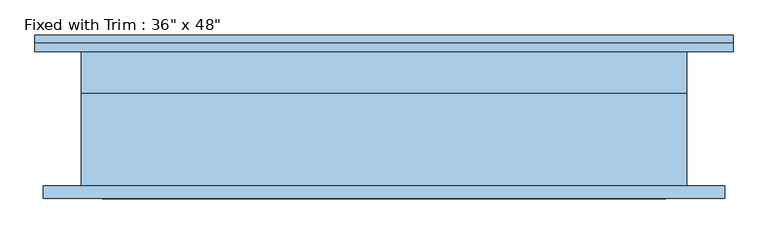
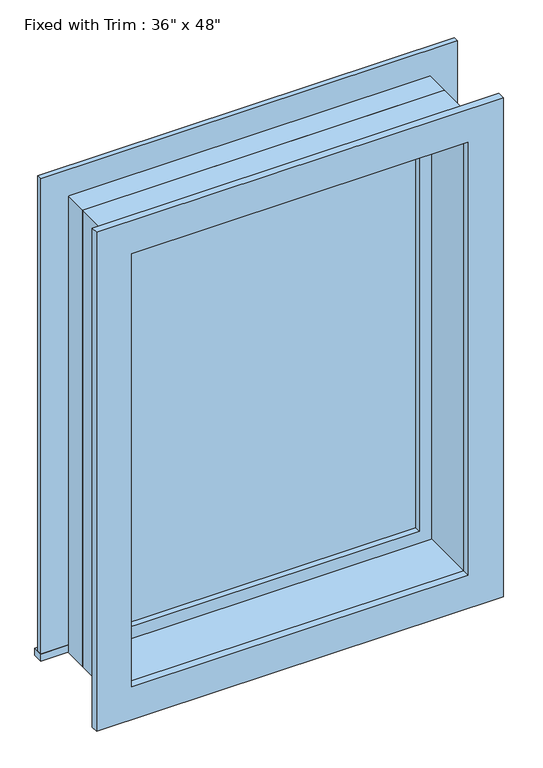
"""IFC4 building model written with IfcOpenShell, lengths in millimetres: window geometry."""

from ifc_helpers import new_model, si_unit, frame, origin, place, context, project, spatial, polyline, outline, extrude, source, transform, mapped, element, save


def window_bec2521a(model_context):
    return source(origin(), model_context, "Body", "SweptSolid", [
        extrude(outline(polyline([(-565.15, 127.0), (488.95, 127.0), (488.95, 101.6), (-565.15, 101.6), (-565.15, 127.0)])), frame((0.0, 0.0, 914.4), z_axis=(0.0, 0.0, 1.0), x_axis=(1.0, 0.0, 0.0)), (0.0, 0.0, 1.0), 19.05),
        extrude(outline(polyline([(2114.55, -476.25), (2114.55, 400.05), (933.45, 400.05), (933.45, 488.95), (2203.45, 488.95), (2203.45, -565.15), (933.45, -565.15), (933.45, -476.25), (2114.55, -476.25)])), frame((0.0, 101.6, 0.0), z_axis=(0.0, 1.0, 0.0), x_axis=(0.0, 0.0, 1.0)), (0.0, 0.0, 1.0), 12.7),
        extrude(outline(polyline([(2190.75, 476.25), (2190.75, -552.45), (857.25, -552.45), (857.25, 476.25), (2190.75, 476.25)]), holes=[polyline([(2101.85, 387.35), (946.15, 387.35), (946.15, -463.55), (2101.85, -463.55), (2101.85, 387.35)])]), frame((0.0, -120.65, 0.0), z_axis=(0.0, 1.0, 0.0), x_axis=(0.0, 0.0, 1.0)), (0.0, 0.0, 1.0), 19.05),
        extrude(outline(polyline([(355.6, 53.975), (-431.8, 53.975), (-431.8, 66.675), (355.6, 66.675), (355.6, 53.975)])), frame((0.0, 0.0, 977.9), z_axis=(0.0, 0.0, 1.0), x_axis=(1.0, 0.0, 0.0)), (0.0, 0.0, 1.0), 1092.2),
        extrude(outline(polyline([(2114.55, -476.25), (933.45, -476.25), (933.45, 400.05), (2114.55, 400.05), (2114.55, -476.25)]), holes=[polyline([(2070.1, -431.8), (2070.1, 355.6), (977.9, 355.6), (977.9, -431.8), (2070.1, -431.8)])]), frame((0.0, 38.1, 0.0), z_axis=(0.0, 1.0, 0.0), x_axis=(0.0, 0.0, 1.0)), (0.0, 0.0, 1.0), 44.45),
        extrude(outline(polyline([(2133.6, -495.3), (914.4, -495.3), (914.4, 419.1), (2133.6, 419.1), (2133.6, -495.3)]), holes=[polyline([(2101.85, -463.55), (2101.85, 387.35), (946.15, 387.35), (946.15, -463.55), (2101.85, -463.55)])]), frame((0.0, -101.6, 0.0), z_axis=(0.0, 1.0, 0.0), x_axis=(0.0, 0.0, 1.0)), (0.0, 0.0, 1.0), 139.7),
        extrude(outline(polyline([(2133.6, 419.1), (2133.6, -495.3), (914.4, -495.3), (914.4, 419.1), (2133.6, 419.1)]), holes=[polyline([(2114.55, 400.05), (933.45, 400.05), (933.45, -476.25), (2114.55, -476.25), (2114.55, 400.05)])]), frame((0.0, 38.1, 0.0), z_axis=(0.0, 1.0, 0.0), x_axis=(0.0, 0.0, 1.0)), (0.0, 0.0, 1.0), 63.5),
    ])


if __name__ == "__main__":
    model = new_model("IFC4")
    model_context = context("Model", 3, world=origin())
    ifc_project = project(units=[si_unit("LENGTHUNIT", "METRE", prefix="MILLI")], contexts=[model_context])
    site = spatial("IfcSite", under=ifc_project)
    building = spatial("IfcBuilding", under=site)
    placement = place(None, origin())
    window_shape = window_bec2521a(model_context)
    element("IfcWindow", 1, ObjectType="Fixed with Trim : 36\" x 48\"", at=placement, inside=building, context=model_context, shape_type="MappedRepresentation", body=[
        mapped(window_shape, transform((0.0, 0.0, 0.0), x_axis=(1.0, 0.0, 0.0), y_axis=(0.0, 1.0, 0.0), z_axis=(0.0, 0.0, 1.0))),
    ])
    save(model, "model.ifc")

# Revit data of these elements
# Type "Fixed with Trim : 36\" x 48\""
#   Type Mark = "10"
#   Construction Type Id = "GSP4R"
#   Assembly Code = "B2020100"
#   Analytic Construction = "1/8 in Pilkington single glazing"
#   Visual Light Transmittance = 0.9
#   Solar Heat Gain Coefficient = 0.78
#   Heat Transfer Coefficient (U) = 0.6496 BTU/(h·ft²·°F)
#   Height = 4' - 0"
#   Default Sill Height = 3' - 0"
#   Trim Projection - Ext. = 0' - 0 1/2"
#   Trim Projection - Int. = 0' - 0 3/4"
#   Trim Width - Exterior = 0' - 3 1/2"
#   Trim Width - Interior = 0' - 3 1/2"
#   Width = 3' - 0"
#   Window Inset = 0' - 0 3/4"
#   Define Thermal Properties by = 1
#   Glass Pane Material = Glass
#   Sash Material = Sash
#   Trim Exterior Material = Trim
#   Trim Interior Material = Trim
#   Wall Closure = (empty or 0)
# Element 1 (IfcWindow, "Fixed with Trim : 36\" x 48\"")
#   Materials on its faces: "Sash", "Trim", "Glass"
# Materials
#   "Glass": class "Glass", colour RGB 0 128 192, transparency 0.75, Description = "Soda Lime Glass", Cost = 0
#   "Sash": class "Wood", colour RGB 224 178 126, transparency 0
#   "Trim": class "Wood", colour RGB 224 178 126, transparency 0
